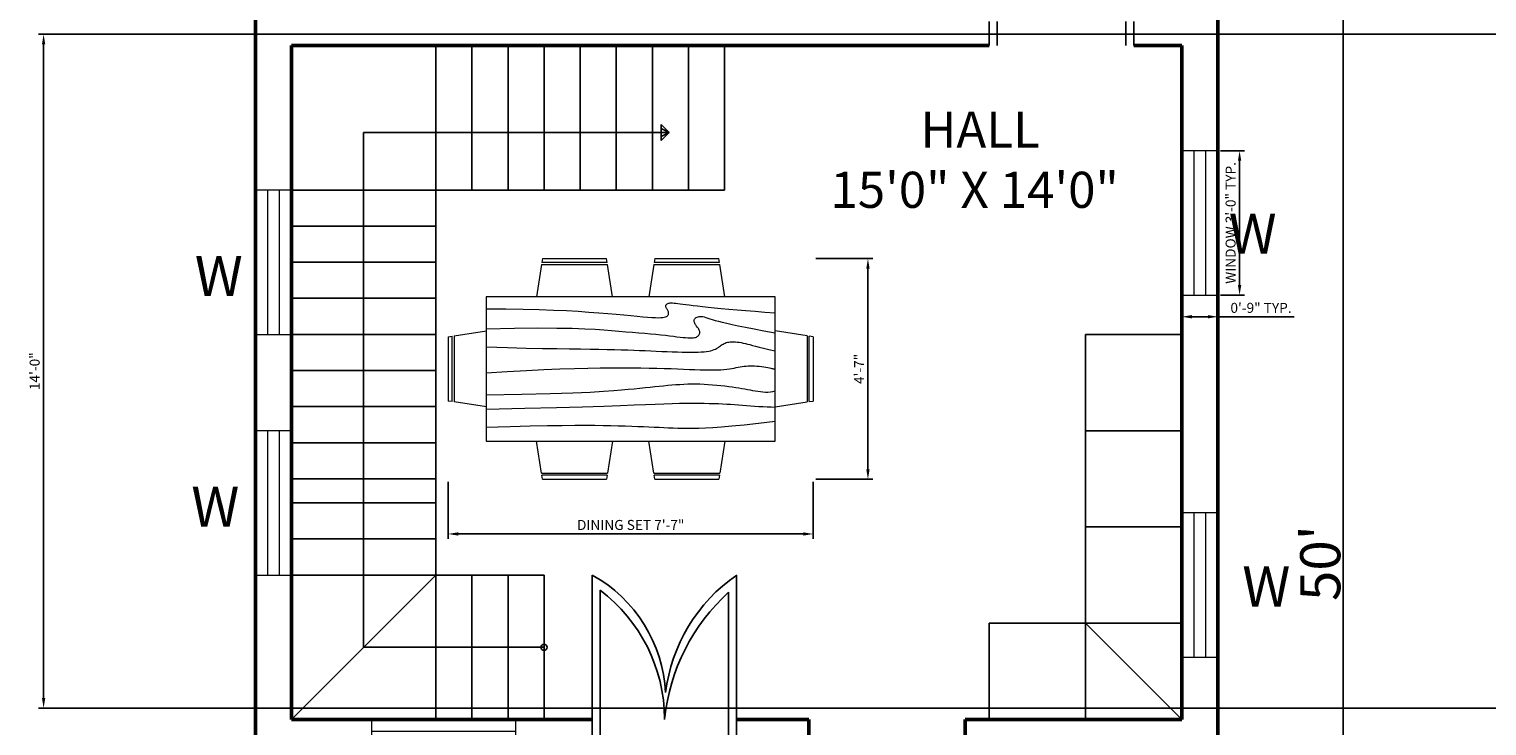
# Model space of a CAD drawing. Units: inches. Extents: x 995 to 2141, y 2161 to 2928.
# Tile 3 of 7: x 995 to 1358, y 2537 to 2711. Entities that reach past the tile are written whole.
import ezdxf

# ---------------------------------------------------------------- set-up
doc = ezdxf.new("R2010")
doc.units = ezdxf.units.IN
for name, color, linetype, lineweight in [('A-ANNO-DIMS', 2, 'Continuous', 18), ('A-ANNO-TEXT', 7, 'Continuous', 18), ('A-AREA-IDEN', 7, 'Continuous', 25), ('A-DOOR', 3, 'Continuous', 25), ('A-FLOR-CASE', 8, 'Continuous', 25), ('A-FLOR-STRS', 7, 'Continuous', 25), ('A-FURN', 8, 'Continuous', 18), ('A-GLAZ', 4, 'Continuous', 18), ('A-WALL', 7, 'Continuous', 50)]:
    doc.layers.add(name, color=color, linetype=linetype, lineweight=lineweight)
doc.styles.get("Standard").update_dxf_attribs({"font": 'arial.ttf'})
doc.dimstyles.new('ISO-25', dxfattribs={"dimtxt": 2.5, "dimasz": 2.5, "dimexe": 1.25, "dimexo": 0.625, "dimtad": 1, "dimdec": 0, "dimlunit": 3, "dimtxsty": 'Standard', "dimcen": 2.5, "dimadec": 0, "dimazin": 0, "dimtfac": 1, "dimtdec": 0, "dimtmove": 0, "dimatfit": 3, "dimfxl": 1, "dimarcsym": 0})

# ---------------------------------------------------------------- blocks, each defined once
blk = doc.blocks.new('Dining Set - 36 x 72 in.')
for p, q in [((-22.2343, 26.00059), (-23.4847, 17.99762)), ((-22.2304, 26), (-5.7608, 26)), ((-22, 27.5), (-22.1562, 26.50042)), ((-5.8416, 26.5), (-22.1534, 26.5)), ((-22, 27.5), (-6, 27.5)), ((-5.8437, 26.49966), (-6, 27.5)), ((-4.5152, 17.99762), (-5.7655, 25.99926)), ((5.7657, 26.00059), (4.5153, 17.99762)), ((5.7696, 26), (22.2392, 26)), ((6, 27.5), (5.8438, 26.50042)), ((22.1584, 26.5), (5.8466, 26.5)), ((6, 27.5), (22, 27.5)), ((22.1563, 26.49966), (22, 27.5)), ((23.4848, 17.99762), (22.2345, 25.99926)), ((36, 18), (-36, 18)), ((-36, 18), (-36, -18)), ((36, -18), (36, 18)), ((-45.5, 8), (-44.5004, 8.15617)), ((-45.5, 8), (-45.5, -8)), ((-44.5, -8.15843), (-44.5, 8.15338)), ((-44.0006, 8.23428), (-35.9976, 9.48474)), ((-44, 8.23041), (-44, -8.23915)), ((44.0006, 8.23428), (35.9976, 9.48474)), ((44, 8.23041), (44, -8.23915)), ((44.5, -8.15843), (44.5, 8.15338)), ((45.5, 8), (44.5005, 8.15617)), ((45.5, 8), (45.5, -8)), ((-44.4997, -8.15631), (-45.5, -8)), ((-35.9976, -9.48476), (-43.9993, -8.2345)), ((35.9976, -9.48476), (43.9993, -8.2345)), ((44.4997, -8.15631), (45.5, -8)), ((-36, -18), (36, -18)), ((-22.2343, -26.0006), (-23.4847, -17.99762)), ((-4.5152, -17.99762), (-5.7655, -25.99928)), ((5.7657, -26.0006), (4.5153, -17.99762)), ((23.4848, -17.99762), (22.2345, -25.99928)), ((-22.2304, -26), (-5.7608, -26)), ((-22, -27.5), (-22.1562, -26.50044)), ((-5.8416, -26.5), (-22.1534, -26.5)), ((-22, -27.5), (-6, -27.5)), ((-5.8437, -26.49967), (-6, -27.5)), ((5.7696, -26), (22.2392, -26)), ((6, -27.5), (5.8438, -26.50044)), ((22.1584, -26.5), (5.8466, -26.5)), ((6, -27.5), (22, -27.5)), ((22.1563, -26.49967), (22, -27.5))]:
    blk.add_line(p, q)
for points in [[(-36, 15), (-31.1772, 14.97754), (-26.8079, 14.91406), (-22.8538, 14.81543), (-19.276, 14.6875), (-16.0362, 14.53613), (-13.0957, 14.36718), (-10.4159, 14.18652), (-7.9583, 14), (-5.6904, 13.81315), (-3.6035, 13.63021), (-1.6954, 13.45508), (0.0365, 13.29166), (1.5945, 13.14388), (2.9811, 13.01562), (4.1988, 12.9108), (5.25, 12.83333), (6.1393, 12.78613), (6.8802, 12.76823), (7.4883, 12.77767), (7.9792, 12.8125), (8.3685, 12.87077), (8.6719, 12.95052), (8.9049, 13.0498), (9.0833, 13.16666), (9.2205, 13.29899), (9.3216, 13.44401), (9.3895, 13.59879), (9.4271, 13.76041), (9.4373, 13.92594), (9.4232, 14.09245), (9.3875, 14.257), (9.3333, 14.41666), (9.2638, 14.56917), (9.1836, 14.71484), (9.0975, 14.85465), (9.0104, 14.98958), (8.9272, 15.1206), (8.8529, 15.2487), (8.7922, 15.37483), (8.75, 15.5), (8.7305, 15.62467), (8.7344, 15.74739), (8.7617, 15.86621), (8.8125, 15.97916), (8.8867, 16.08431), (8.9844, 16.17968), (9.1055, 16.26334), (9.25, 16.33333), (9.4189, 16.38802), (9.6172, 16.42708), (9.8506, 16.45052), (10.125, 16.45833), (10.4463, 16.45052), (10.8203, 16.42708), (11.2529, 16.38802), (11.75, 16.33333), (12.3184, 16.26318), (12.9694, 16.17838), (13.7151, 16.07991), (14.5677, 15.96875), (15.5395, 15.84586), (16.6426, 15.71224), (17.8893, 15.56884), (19.2917, 15.41666), (20.859, 15.25667), (22.5879, 15.08984), (24.4721, 14.91715), (26.5052, 14.73958), (28.6809, 14.5581), (30.9929, 14.3737), (33.4347, 14.18733), (36, 14)], [(-36, 10), (-28.9766, 10.14274), (-23.1725, 10.20442), (-18.4241, 10.19775), (-14.5677, 10.13541), (-11.4399, 10.03011), (-8.877, 9.89453), (-6.7154, 9.74137), (-4.7917, 9.58333), (-2.9698, 9.43082), (-1.2246, 9.28515), (0.4415, 9.14534), (2.026, 9.01041), (3.5266, 8.87939), (4.9408, 8.7513), (6.266, 8.62516), (7.5, 8.5), (8.6411, 8.37549), (9.6914, 8.2539), (10.6538, 8.13818), (11.5312, 8.03125), (12.3267, 7.93603), (13.043, 7.85547), (13.6831, 7.79248), (14.25, 7.75), (14.7471, 7.7303), (15.1797, 7.73307), (15.5537, 7.75732), (15.875, 7.80208), (16.1494, 7.86637), (16.3828, 7.94922), (16.5811, 8.04964), (16.75, 8.16666), (16.8944, 8.29915), (17.0143, 8.44531), (17.1089, 8.60319), (17.1771, 8.77083), (17.218, 8.94629), (17.2305, 9.1276), (17.2137, 9.31282), (17.1667, 9.5), (17.0895, 9.6875), (16.987, 9.875), (16.8649, 10.0625), (16.7292, 10.25), (16.5856, 10.4375), (16.4401, 10.625), (16.2985, 10.8125), (16.1667, 11), (16.05, 11.18733), (15.9518, 11.3737), (15.8752, 11.5581), (15.8229, 11.73958), (15.798, 11.91715), (15.8034, 12.08984), (15.842, 12.25667), (15.9167, 12.41666), (16.0295, 12.56836), (16.1784, 12.70833), (16.3605, 12.83268), (16.5729, 12.9375), (16.8127, 13.01888), (17.0768, 13.07291), (17.3625, 13.0957), (17.6667, 13.08333), (17.9894, 13.03312), (18.3418, 12.94726), (18.7382, 12.82918), (19.1927, 12.68229), (19.7195, 12.51001), (20.3327, 12.31575), (21.0465, 12.10294), (21.875, 11.875), (22.8357, 11.63354), (23.959, 11.37304), (25.2786, 11.08618), (26.8282, 10.76562), (28.6414, 10.40405), (30.752, 9.99414), (33.1936, 9.52856), (36, 9)], [(-36, 5.5), (-30.7157, 5.3348), (-26.069, 5.20963), (-21.9946, 5.11767), (-18.4271, 5.05208), (-15.3009, 5.00602), (-12.5508, 4.97265), (-10.1112, 4.94515), (-7.9167, 4.91666), (-5.909, 4.88167), (-4.0586, 4.83984), (-2.3429, 4.79215), (-0.7396, 4.73958), (0.7739, 4.6831), (2.22, 4.6237), (3.6213, 4.56233), (5, 4.5), (6.373, 4.43782), (7.7344, 4.3776), (9.0723, 4.32129), (10.375, 4.27083), (11.6309, 4.22819), (12.8281, 4.19531), (13.9551, 4.17415), (15, 4.16666), (15.954, 4.17448), (16.819, 4.19791), (17.6001, 4.23698), (18.3021, 4.29166), (18.9299, 4.36198), (19.4883, 4.44791), (19.9823, 4.54948), (20.4167, 4.66666), (20.7969, 4.79899), (21.1302, 4.94401), (21.4245, 5.09879), (21.6875, 5.26041), (21.9271, 5.42594), (22.1511, 5.59245), (22.3672, 5.757), (22.5834, 5.91666), (22.8065, 6.06868), (23.0404, 6.21093), (23.2879, 6.34147), (23.5521, 6.45833), (23.8358, 6.55957), (24.142, 6.64323), (24.4735, 6.70735), (24.8334, 6.75), (25.2235, 6.76969), (25.642, 6.76692), (26.0858, 6.74267), (26.5521, 6.69791), (27.0379, 6.63362), (27.5404, 6.55078), (28.0565, 6.45036), (28.5834, 6.33333), (29.1242, 6.19987), (29.7071, 6.04687), (30.3661, 5.87044), (31.1354, 5.66666), (32.0493, 5.43164), (33.142, 5.16146), (34.4475, 4.85221), (36, 4.5)], [(-36, -1), (-30.7915, -0.6591), (-26.0195, -0.38216), (-21.6519, -0.16284), (-17.6563, 0.00521), (-14.0005, 0.12833), (-10.6523, 0.21289), (-7.5796, 0.26522), (-4.75, 0.29166), (-2.134, 0.29793), (0.2878, 0.28711), (2.5317, 0.26163), (4.6146, 0.22396), (6.5529, 0.17651), (8.3633, 0.12174), (10.0623, 0.06209), (11.6667, 0), (13.1899, -0.06201), (14.6341, -0.1211), (15.9982, -0.17432), (17.2813, -0.21875), (18.4823, -0.25147), (19.6003, -0.26953), (20.6343, -0.27002), (21.5834, -0.25), (22.4481, -0.20768), (23.2357, -0.14584), (23.9549, -0.06836), (24.6146, 0.02083), (25.2235, 0.11784), (25.7904, 0.21875), (26.3241, 0.31966), (26.8334, 0.41666), (27.3265, 0.50618), (27.8099, 0.58593), (28.2894, 0.65397), (28.7709, 0.70833), (29.2601, 0.74707), (29.763, 0.76823), (30.2855, 0.76985), (30.8334, 0.75), (31.4088, 0.70784), (31.9994, 0.64713), (32.589, 0.57275), (33.1615, 0.48958), (33.7008, 0.4025), (34.1908, 0.3164), (34.6153, 0.23616), (34.9584, 0.16666), (35.2099, 0.11165), (35.3848, 0.07031), (35.504, 0.04069), (35.5886, 0.02083), (35.6594, 0.00879), (35.7377, 0.0026), (35.8442, 0.00032), (36, 0)], [(-36, -6.5), (-27.1843, -6.31267), (-20.084, -6.1263), (-14.469, -5.9419), (-10.1094, -5.76042), (-6.7752, -5.58285), (-4.2363, -5.41016), (-2.2629, -5.24333), (-0.625, -5.08334), (0.8708, -4.93099), (2.2715, -4.78646), (3.5872, -4.64974), (4.8281, -4.52084), (6.0046, -4.39974), (7.127, -4.28646), (8.2053, -4.18099), (9.25, -4.08334), (10.2705, -3.99382), (11.2734, -3.91407), (12.2647, -3.84603), (13.25, -3.79167), (14.2354, -3.75293), (15.2266, -3.73177), (16.2295, -3.73015), (17.25, -3.75), (18.2912, -3.79248), (19.3451, -3.85547), (20.4009, -3.93604), (21.4479, -4.03125), (22.4754, -4.13819), (23.4727, -4.25391), (24.4289, -4.37549), (25.3334, -4.5), (26.1785, -4.62492), (26.9694, -4.74935), (27.7145, -4.87281), (28.4219, -4.99479), (29.1, -5.11483), (29.7572, -5.23242), (30.4016, -5.34709), (31.0417, -5.45834), (31.6837, -5.56437), (32.3262, -5.65821), (32.9658, -5.73153), (33.599, -5.77604), (34.2224, -5.78345), (34.8327, -5.74545), (35.4264, -5.65373), (36, -5.5)], [(-36, -10), (-26.4022, -9.81299), (-18.4675, -9.62891), (-11.9839, -9.45069), (-6.7396, -9.28125), (-2.5226, -9.12354), (0.8789, -8.98047), (3.6769, -8.85498), (6.0833, -8.75), (8.2767, -8.66765), (10.3021, -8.60677), (12.1712, -8.56543), (13.8958, -8.54167), (15.4876, -8.53353), (16.9583, -8.53907), (18.3197, -8.55632), (19.5834, -8.58334), (20.7616, -8.61841), (21.8685, -8.66081), (22.9188, -8.71004), (23.9271, -8.76563), (24.9081, -8.82707), (25.8763, -8.89388), (26.8465, -8.96558), (27.8334, -9.04167), (28.8474, -9.12118), (29.8828, -9.20117), (30.93, -9.27824), (31.9792, -9.34896), (33.0205, -9.40991), (34.0443, -9.45768), (35.0407, -9.48885), (36, -9.5)], [(-36, -14.5), (-30.0881, -14.33513), (-25.0332, -14.21224), (-20.7312, -14.12647), (-17.0781, -14.07292), (-13.97, -14.04671), (-11.3027, -14.04297), (-8.9724, -14.05681), (-6.875, -14.08334), (-4.9224, -14.11833), (-3.0905, -14.16016), (-1.3709, -14.20785), (0.2448, -14.26042), (1.7647, -14.3169), (3.1973, -14.3763), (4.5507, -14.43767), (5.8333, -14.5), (7.0554, -14.5621), (8.235, -14.62175), (9.3922, -14.67652), (10.5469, -14.72396), (11.7192, -14.76164), (12.929, -14.78711), (14.1965, -14.79794), (15.5417, -14.79167), (16.9933, -14.76424), (18.6152, -14.70508), (20.4804, -14.60197), (22.6615, -14.44271), (25.2312, -14.21509), (28.2624, -13.9069), (31.8277, -13.50594), (36, -13)]]:
    blk.add_lwpolyline(points)
blk = doc.blocks.new('*D17')
at = {"layer": 'A-ANNO-DIMS', "color": 0, "lineweight": -2, "transparency": 16777216}
for p, q in [((1291.61, 2877.69), (1323.48, 2877.69)), ((1322.23, 2875.19), (1322.23, 2280.19)), ((1291.61, 2277.69), (1323.48, 2277.69))]:
    blk.add_line(p, q, dxfattribs=at)
at = {"layer": 'A-ANNO-DIMS', "color": 0, "transparency": 16777216}
for points in [[(1321.81, 2875.19), (1322.65, 2875.19), (1322.23, 2877.69)], [(1321.81, 2280.19), (1322.65, 2280.19), (1322.23, 2277.69)]]:
    blk.add_solid(points, dxfattribs=at)
at = {"layer": 'Defpoints', "color": 0, "transparency": 16777216}
for p in [(1290.98, 2877.69), (1290.98, 2277.69), (1322.23, 2277.69)]:
    blk.add_point(p, dxfattribs=at)
at = {"layer": 'A-ANNO-DIMS', "color": 0, "transparency": 16777216, "insert": (1316.5, 2577.69), "char_height": 2.5, "attachment_point": 5, "rotation": 90}
blk.add_mtext("{\\H4x;50'}", dxfattribs=at)
blk = doc.blocks.new('WIN-36IN')
for p, q in [((0, 36), (0, 0)), ((9, 36), (0, 36)), ((3, 36), (3, 0)), ((6, 0), (6, 36)), ((9, 0), (9, 36)), ((0, 0), (9, 0))]:
    blk.add_line(p, q)
blk = doc.blocks.new('*D30')
at = {"layer": 'A-ANNO-DIMS', "color": 0, "lineweight": -2, "transparency": 16777216}
for p, q in [((1291.61, 2680.49), (1297.63, 2680.49)), ((1296.38, 2646.99), (1296.38, 2677.99)), ((1291.61, 2644.49), (1297.63, 2644.49))]:
    blk.add_line(p, q, dxfattribs=at)
at = {"layer": 'A-ANNO-DIMS', "color": 0, "transparency": 16777216}
for points in [[(1295.97, 2677.99), (1296.8, 2677.99), (1296.38, 2680.49)], [(1295.97, 2646.99), (1296.8, 2646.99), (1296.38, 2644.49)]]:
    blk.add_solid(points, dxfattribs=at)
at = {"layer": 'Defpoints', "color": 0, "transparency": 16777216}
for p in [(1290.98, 2680.49), (1296.38, 2680.49), (1290.98, 2644.49)]:
    blk.add_point(p, dxfattribs=at)
at = {"layer": 'A-ANNO-DIMS', "color": 0, "transparency": 16777216, "insert": (1294.47, 2662.49), "char_height": 2.5, "attachment_point": 5, "rotation": 90}
blk.add_mtext('WINDOW 3\'-0" TYP.', dxfattribs=at)
blk = doc.blocks.new('*D31')
at = {"layer": 'A-ANNO-DIMS', "color": 0, "lineweight": -2, "transparency": 16777216}
for p, q in [((1281.98, 2643.87), (1281.98, 2637.84)), ((1290.98, 2643.87), (1290.98, 2637.84)), ((1284.48, 2639.09), (1288.48, 2639.09)), ((1290.98, 2639.09), (1309.97, 2639.09))]:
    blk.add_line(p, q, dxfattribs=at)
at = {"layer": 'A-ANNO-DIMS', "color": 0, "transparency": 16777216}
for points in [[(1284.48, 2639.51), (1284.48, 2638.68), (1281.98, 2639.09)], [(1288.48, 2639.51), (1288.48, 2638.68), (1290.98, 2639.09)]]:
    blk.add_solid(points, dxfattribs=at)
at = {"layer": 'Defpoints', "color": 0, "transparency": 16777216}
for p in [(1281.98, 2644.49), (1290.98, 2644.49), (1290.98, 2639.09)]:
    blk.add_point(p, dxfattribs=at)
at = {"layer": 'A-ANNO-DIMS', "color": 0, "transparency": 16777216, "insert": (1301.73, 2640.99), "char_height": 2.5, "attachment_point": 5}
blk.add_mtext('0\'-9" TYP.', dxfattribs=at)
blk = doc.blocks.new('*D52')
at = {"layer": 'A-ANNO-DIMS', "color": 0, "lineweight": -2, "transparency": 16777216}
for p, q in [((1099.07, 2597.97), (1099.07, 2583.69)), ((1190.07, 2597.97), (1190.07, 2583.69)), ((1101.57, 2584.94), (1187.57, 2584.94))]:
    blk.add_line(p, q, dxfattribs=at)
at = {"layer": 'A-ANNO-DIMS', "color": 0, "transparency": 16777216}
for points in [[(1101.57, 2585.36), (1101.57, 2584.53), (1099.07, 2584.94)], [(1187.57, 2585.36), (1187.57, 2584.53), (1190.07, 2584.94)]]:
    blk.add_solid(points, dxfattribs=at)
at = {"layer": 'Defpoints', "color": 0, "transparency": 16777216}
for p in [(1099.07, 2598.59), (1190.07, 2598.59), (1190.07, 2584.94)]:
    blk.add_point(p, dxfattribs=at)
at = {"layer": 'A-ANNO-DIMS', "color": 0, "transparency": 16777216, "insert": (1144.57, 2586.86), "char_height": 2.5, "attachment_point": 5}
blk.add_mtext('DINING SET 7\'-7"', dxfattribs=at)
blk = doc.blocks.new('*D53')
at = {"layer": 'A-ANNO-DIMS', "color": 0, "lineweight": -2, "transparency": 16777216}
for p, q in [((1190.7, 2653.59), (1204.97, 2653.59)), ((1203.72, 2601.09), (1203.72, 2651.09)), ((1190.7, 2598.59), (1204.97, 2598.59))]:
    blk.add_line(p, q, dxfattribs=at)
at = {"layer": 'A-ANNO-DIMS', "color": 0, "transparency": 16777216}
for points in [[(1203.3, 2651.09), (1204.14, 2651.09), (1203.72, 2653.59)], [(1203.3, 2601.09), (1204.14, 2601.09), (1203.72, 2598.59)]]:
    blk.add_solid(points, dxfattribs=at)
at = {"layer": 'Defpoints', "color": 0, "transparency": 16777216}
for p in [(1190.07, 2653.59), (1203.72, 2653.59), (1190.07, 2598.59)]:
    blk.add_point(p, dxfattribs=at)
at = {"layer": 'A-ANNO-DIMS', "color": 0, "transparency": 16777216, "insert": (1201.85, 2626.09), "char_height": 2.5, "attachment_point": 5, "rotation": 90}
blk.add_mtext('4\'-7"', dxfattribs=at)
blk = doc.blocks.new('*D65')
at = {"layer": 'A-ANNO-DIMS', "color": 0, "lineweight": -2, "transparency": 16777216}
for p, q in [((1441.38, 2709.52), (996.93, 2709.52)), ((998.18, 2544.02), (998.18, 2707.02)), ((1441.38, 2541.52), (996.93, 2541.52))]:
    blk.add_line(p, q, dxfattribs=at)
at = {"layer": 'A-ANNO-DIMS', "color": 0, "transparency": 16777216}
for points in [[(997.77, 2707.02), (998.6, 2707.02), (998.18, 2709.52)], [(997.77, 2544.02), (998.6, 2544.02), (998.18, 2541.52)]]:
    blk.add_solid(points, dxfattribs=at)
at = {"layer": 'Defpoints', "color": 0, "transparency": 16777216}
for p in [(998.18, 2709.52), (1442, 2709.52), (1442, 2541.52)]:
    blk.add_point(p, dxfattribs=at)
at = {"layer": 'A-ANNO-DIMS', "color": 0, "transparency": 16777216, "insert": (996.28, 2625.52), "char_height": 2.5, "attachment_point": 5, "rotation": 90}
blk.add_mtext('14\'-0"', dxfattribs=at)

msp = doc.modelspace()

# ---------------------------------------------------------------- linework, layer by layer
at = {"layer": 'A-DOOR'}
for p, q in [((1233.98, 2706.69), (1233.98, 2712.69)), ((1235.98, 2706.69), (1235.98, 2712.69)), ((1267.98, 2712.69), (1267.98, 2706.69)), ((1269.98, 2712.69), (1269.98, 2706.69)), ((1134.98, 2538.69), (1134.98, 2574.69)), ((1170.98, 2538.69), (1170.98, 2574.69)), ((1136.98, 2538.69), (1136.98, 2570.89)), ((1168.98, 2538.69), (1168.98, 2570.42)), ((1134.98, 2538.69), (1134.98, 2532.69)), ((1136.98, 2538.69), (1136.98, 2532.69)), ((1168.98, 2532.69), (1168.98, 2538.69)), ((1170.98, 2532.69), (1170.98, 2538.69))]:
    msp.add_line(p, q, dxfattribs=at)
for centre, radius, start, end in [((1117.63, 2543.51), 35.69, 3.0018, 60.8945), ((1194.76, 2540.3), 41.8, 124.6579, 173.0254), ((1112.49, 2538.59), 40.54, 0.5201, 52.8171), ((1202.36, 2533.71), 49.62, 132.2719, 173.9214), ((1117.63, 2543.51), 35.69, 352.2356, 354.0438)]:
    msp.add_arc(centre, radius, start, end, dxfattribs=at)
at = {"layer": 'A-FLOR-CASE'}
for p, q in [((1257.98, 2634.69), (1257.98, 2538.69)), ((1257.98, 2634.69), (1281.98, 2634.69)), ((1257.98, 2610.69), (1281.98, 2610.69)), ((1257.98, 2586.69), (1281.98, 2586.69)), ((1233.98, 2562.69), (1233.98, 2538.69)), ((1257.98, 2562.69), (1233.98, 2562.69)), ((1257.98, 2562.69), (1281.98, 2562.69)), ((1257.98, 2562.69), (1281.98, 2538.69))]:
    msp.add_line(p, q, dxfattribs=at)
at = {"layer": 'A-FLOR-STRS'}
for p, q in [((1095.98, 2538.69), (1095.98, 2706.69)), ((1104.98, 2670.69), (1104.98, 2706.69)), ((1113.98, 2670.69), (1113.98, 2706.69)), ((1122.98, 2670.69), (1122.98, 2706.69)), ((1131.98, 2670.69), (1131.98, 2706.69)), ((1140.98, 2670.69), (1140.98, 2706.69)), ((1149.98, 2670.69), (1149.98, 2706.69)), ((1158.98, 2670.69), (1158.98, 2706.69)), ((1167.98, 2670.69), (1167.98, 2706.69)), ((1152.19, 2685.02), (1152.19, 2687.02)), ((1152.19, 2687.02), (1152.19, 2685.02)), ((1154.19, 2685.02), (1152.19, 2687.02)), ((1152.19, 2687.02), (1154.19, 2685.02)), ((1154.19, 2685.02), (1152.19, 2686.02)), ((1077.98, 2556.69), (1077.98, 2685.02)), ((1077.98, 2685.02), (1079.98, 2685.02)), ((1079.98, 2685.02), (1152.19, 2685.02)), ((1152.19, 2685.02), (1152.19, 2683.02)), ((1152.19, 2683.02), (1152.19, 2685.02)), ((1152.19, 2685.02), (1154.19, 2685.02)), ((1154.19, 2685.02), (1152.19, 2683.02)), ((1152.19, 2684.02), (1154.19, 2685.02)), ((1152.19, 2683.02), (1152.19, 2684.02)), ((1059.98, 2670.69), (1167.98, 2670.69)), ((1059.98, 2661.69), (1095.98, 2661.69)), ((1059.98, 2652.69), (1095.98, 2652.69)), ((1059.98, 2643.69), (1095.98, 2643.69)), ((1059.98, 2634.69), (1095.98, 2634.69)), ((1059.98, 2625.69), (1095.98, 2625.69)), ((1059.98, 2616.69), (1095.98, 2616.69)), ((1059.98, 2607.69), (1095.98, 2607.69)), ((1059.98, 2607.69), (1095.98, 2607.69)), ((1059.98, 2607.69), (1095.98, 2607.69)), ((1059.98, 2598.69), (1095.98, 2598.69)), ((1059.98, 2592.69), (1095.98, 2592.69)), ((1059.98, 2583.69), (1095.98, 2583.69)), ((1059.98, 2574.69), (1122.98, 2574.69)), ((1059.98, 2574.69), (1122.98, 2574.69)), ((1095.98, 2574.69), (1059.98, 2538.69)), ((1104.98, 2538.69), (1104.98, 2574.69)), ((1113.98, 2538.69), (1113.98, 2574.69)), ((1122.98, 2538.69), (1122.98, 2574.69)), ((1122.98, 2556.69), (1077.98, 2556.69))]:
    msp.add_line(p, q, dxfattribs=at)
msp.add_circle((1122.98, 2556.7), 0.765, dxfattribs=at)
at = {"layer": 'A-WALL'}
for p, q in [((1050.98, 2277.69), (1050.98, 2877.69)), ((1290.98, 2877.69), (1290.98, 2277.69)), ((1059.98, 2706.69), (1233.98, 2706.69)), ((1059.98, 2538.69), (1059.98, 2706.69)), ((1269.98, 2706.69), (1281.98, 2706.69)), ((1281.98, 2706.69), (1281.98, 2538.69)), ((1059.98, 2538.69), (1134.98, 2538.69)), ((1170.98, 2538.69), (1188.98, 2538.69)), ((1188.98, 2532.69), (1188.98, 2538.69)), ((1227.98, 2532.69), (1227.98, 2538.69)), ((1227.98, 2538.69), (1281.98, 2538.69))]:
    msp.add_line(p, q, dxfattribs=at)

# ---------------------------------------------------------------- block references
at = {"layer": 'A-FURN'}
msp.add_blockref('Dining Set - 36 x 72 in.', (1144.57, 2626.09), dxfattribs=at)
at = {"layer": 'A-GLAZ'}
for p in [(1281.98, 2644.49), (1050.98, 2634.69), (1050.98, 2574.69), (1281.98, 2554.25)]:
    msp.add_blockref('WIN-36IN', p, dxfattribs=at)
at = {"layer": 'A-GLAZ', "rotation": 269.9999999999986}
msp.add_blockref('WIN-36IN', (1079.93, 2538.69), dxfattribs=at)

# ---------------------------------------------------------------- texts
at = {"layer": 'A-ANNO-TEXT', "char_height": 10, "attachment_point": 1}
for insert in [(1293.66, 2664.83), (1035.87, 2654.26), (1035.01, 2596.73), (1297.06, 2576.85)]:
    msp.add_mtext_dynamic_manual_height_columns('W', width=112.484, gutter_width=12.5, heights=[0], dxfattribs=dict(at, insert=insert))
at = {"layer": 'A-AREA-IDEN', "insert": (1178.66, 2690.25), "char_height": 9, "attachment_point": 1}
msp.add_mtext_dynamic_manual_height_columns('\\pxqc; HALL \\P15\'0" X 14\'0"', width=103.3264, gutter_width=12.5, heights=[0], dxfattribs=at)

# ---------------------------------------------------------------- dimensions: what is measured, and where the dimension line sits
at = {"layer": 'A-ANNO-DIMS'}
for base, p1, p2, text, override, picture, middle in [((1322.23, 2277.69), (1290.98, 2877.69), (1290.98, 2277.69), "{\\H4x;50'}", {"dimclrd": 0, "dimclre": 0, "dimclrt": 0}, '*D17', (1316.5, 2577.69)), ((1296.38, 2680.49), (1290.98, 2644.49), (1290.98, 2680.49), 'WINDOW <> TYP.', {"dimdec": 1, "dimlfac": 1, "dimrnd": 0, "dimzin": 1, "dimdsep": 46, "dimlunit": 4, "dimfrac": 2}, '*D30', (1294.47, 2662.49))]:
    dim = msp.add_linear_dim(base=base, p1=p1, p2=p2, angle=90, text=text, dimstyle='ISO-25', override=override, dxfattribs=at)
    dim.commit()
    dim.dimension.update_dxf_attribs({"geometry": picture, "text_midpoint": middle})
for base, p1, p2, picture, middle in [((998.18, 2709.52), (1442, 2541.52), (1442, 2709.52), '*D65', (996.28, 2625.52)), ((1203.72, 2653.59), (1190.07, 2598.59), (1190.07, 2653.59), '*D53', (1201.85, 2626.09))]:
    dim = msp.add_linear_dim(base=base, p1=p1, p2=p2, angle=90, dimstyle='ISO-25', override={"dimdec": 1, "dimlfac": 1, "dimrnd": 0, "dimzin": 1, "dimdsep": 46, "dimlunit": 4, "dimfrac": 2}, dxfattribs=at)
    dim.commit()
    dim.dimension.update_dxf_attribs({"geometry": picture, "text_midpoint": middle})
for base, p1, p2, text, picture, middle in [((1290.98, 2639.09), (1281.98, 2644.49), (1290.98, 2644.49), '<> TYP.', '*D31', (1301.73, 2640.99)), ((1190.07, 2584.94), (1099.07, 2598.59), (1190.07, 2598.59), 'DINING SET <>', '*D52', (1144.57, 2586.86))]:
    dim = msp.add_linear_dim(base=base, p1=p1, p2=p2, text=text, dimstyle='ISO-25', override={"dimdec": 1, "dimlfac": 1, "dimrnd": 0, "dimzin": 1, "dimdsep": 46, "dimlunit": 4, "dimfrac": 2}, dxfattribs=at)
    dim.commit()
    dim.dimension.update_dxf_attribs({"geometry": picture, "text_midpoint": middle})

doc.saveas('drawing.dxf')
